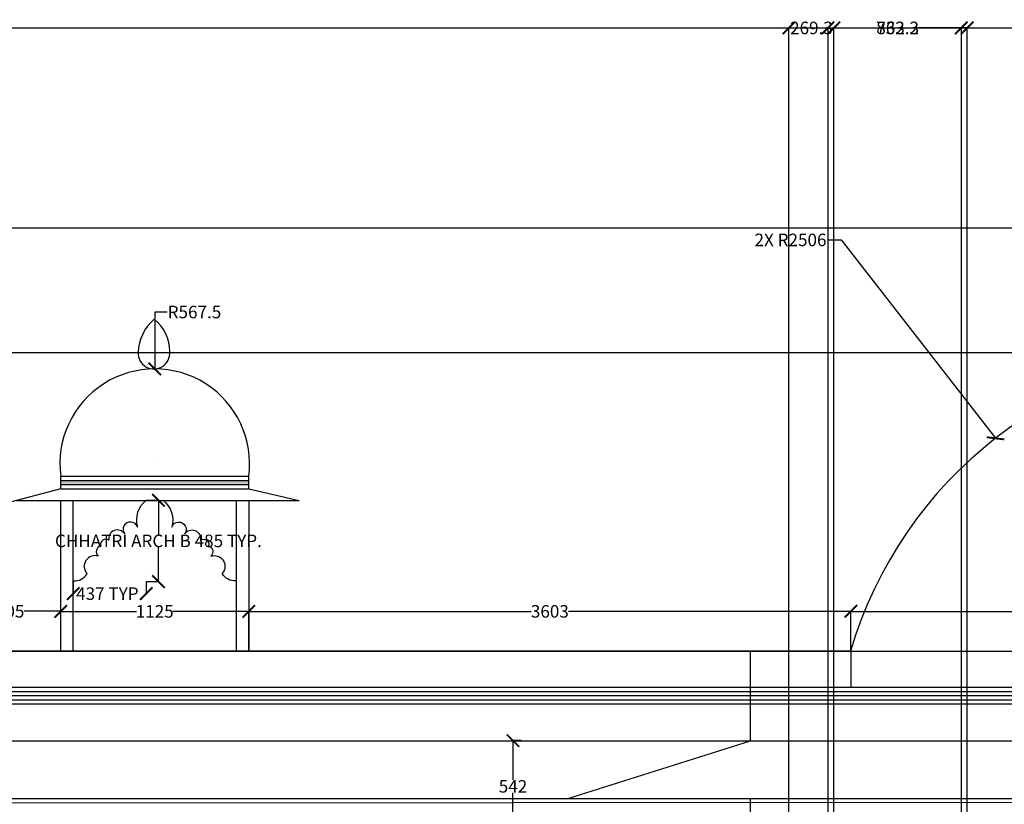
# Model space of a CAD drawing. Units: inches. Extents: x 829 to 33356404, y 1874 to 16983.
# Tile 5 of 9: x 4957 to 10848, y 12288 to 16983. Entities that reach past the tile are written whole.
import ezdxf

# ---------------------------------------------------------------- set-up
doc = ezdxf.new("R2010")
doc.units = ezdxf.units.IN
doc.header["$MEASUREMENT"] = 0
doc.header["$PDMODE"] = 3
for name, color, linetype, lineweight in [('A-ANNO-DIMS', 2, 'Continuous', 18), ('A-ELEV', 7, 'Continuous', 25), ('A-ELEV-PATT', 8, 'Continuous', 13)]:
    doc.layers.add(name, color=color, linetype=linetype, lineweight=lineweight)
doc.styles.get("Standard").update_dxf_attribs({"font": 'arial.ttf'})
doc.dimstyles.get("Standard").update_dxf_attribs({"dimtxt": 75, "dimasz": 75, "dimexe": 0.18, "dimexo": 0.0625, "dimgap": 0.09, "dimtad": 0, "dimtih": 1, "dimtoh": 1, "dimdec": 0, "dimzin": 0, "dimdsep": 46, "dimtxsty": 'Standard', "dimblk": 'ARCHTICK', "dimcen": 0.09, "dimadec": 0, "dimazin": 0, "dimtfac": 1, "dimtdec": 0, "dimtofl": 0, "dimtmove": 0, "dimatfit": 3, "dimfxl": 1, "dimtolj": 1, "dimtzin": 0, "dimarcsym": 0})

# ---------------------------------------------------------------- blocks, each defined once
blk = doc.blocks.new('_ArchTick')
at = {"color": 0, "linetype": 'ByBlock', "const_width": 0.15}
blk.add_lwpolyline([(-0.5, -0.5), (0.5, 0.5)], dxfattribs=at)
blk = doc.blocks.new('*D35')
at = {"layer": 'A-ANNO-DIMS', "color": 0, "lineweight": -2, "transparency": 16777216}
for p, q in [((7957.3, 12669.2), (7908.7, 12669.2)), ((7908.8, 12669.2), (7908.8, 12434.2)), ((7908.8, 12127.2), (7908.8, 12357.4)), ((7957.3, 12127.2), (7908.7, 12127.2))]:
    blk.add_line(p, q, dxfattribs=at)
at = {"layer": 'Defpoints', "color": 0, "transparency": 16777216}
for p in [(7908.8, 12669.2), (7957.3, 12669.2), (7957.3, 12127.2)]:
    blk.add_point(p, dxfattribs=at)
at = {"layer": 'A-ANNO-DIMS', "color": 0, "lineweight": -2, "transparency": 16777216, "xscale": 75, "yscale": 75, "zscale": 75}
for p, rotation in [((7908.8, 12669.2), 90), ((7908.8, 12127.2), 270)]:
    blk.add_blockref('_ArchTick', p, dxfattribs=dict(at, rotation=rotation))
at = {"layer": 'A-ANNO-DIMS', "color": 0, "transparency": 16777216, "insert": (7908.8, 12395.8), "char_height": 75, "attachment_point": 5}
blk.add_mtext('\\A1;542', dxfattribs=at)
blk = doc.blocks.new('*D47')
at = {"layer": 'A-ANNO-DIMS', "color": 0, "lineweight": -2, "transparency": 16777216}
for p, q in [((4597.8, 13204.1), (4597.8, 13443.2)), ((4597.8, 13443), (4816.8, 13443)), ((5202.8, 13443), (4983.7, 13443)), ((5202.8, 13204.1), (5202.8, 13443.2))]:
    blk.add_line(p, q, dxfattribs=at)
at = {"layer": 'Defpoints', "color": 0, "transparency": 16777216}
for p in [(5202.8, 13443), (4597.8, 13204), (5202.8, 13204)]:
    blk.add_point(p, dxfattribs=at)
at = {"layer": 'A-ANNO-DIMS', "color": 0, "lineweight": -2, "transparency": 16777216, "xscale": 75, "yscale": 75, "zscale": 75, "rotation": 180}
blk.add_blockref('_ArchTick', (4597.8, 13443), dxfattribs=at)
at = {"layer": 'A-ANNO-DIMS', "color": 0, "lineweight": -2, "transparency": 16777216, "xscale": 75, "yscale": 75, "zscale": 75}
blk.add_blockref('_ArchTick', (5202.8, 13443), dxfattribs=at)
at = {"layer": 'A-ANNO-DIMS', "color": 0, "transparency": 16777216, "insert": (4900.3, 13443), "char_height": 75, "attachment_point": 5}
blk.add_mtext('\\A1;605', dxfattribs=at)
blk = doc.blocks.new('*D48')
at = {"layer": 'A-ANNO-DIMS', "color": 0, "lineweight": -2, "transparency": 16777216}
for p, q in [((5202.8, 13273.1), (5202.8, 13442.8)), ((5202.8, 13442.7), (5656.4, 13442.7)), ((6327.8, 13442.7), (5874.1, 13442.7)), ((6327.8, 13273.1), (6327.8, 13442.8))]:
    blk.add_line(p, q, dxfattribs=at)
at = {"layer": 'Defpoints', "color": 0, "transparency": 16777216}
for p in [(6327.8, 13442.7), (5202.8, 13273), (6327.8, 13273)]:
    blk.add_point(p, dxfattribs=at)
at = {"layer": 'A-ANNO-DIMS', "color": 0, "lineweight": -2, "transparency": 16777216, "xscale": 75, "yscale": 75, "zscale": 75, "rotation": 180}
blk.add_blockref('_ArchTick', (5202.8, 13442.7), dxfattribs=at)
at = {"layer": 'A-ANNO-DIMS', "color": 0, "lineweight": -2, "transparency": 16777216, "xscale": 75, "yscale": 75, "zscale": 75}
blk.add_blockref('_ArchTick', (6327.8, 13442.7), dxfattribs=at)
at = {"layer": 'A-ANNO-DIMS', "color": 0, "transparency": 16777216, "insert": (5765.3, 13442.7), "char_height": 75, "attachment_point": 5}
blk.add_mtext('\\A1;1125', dxfattribs=at)
blk = doc.blocks.new('*D54')
at = {"layer": 'A-ANNO-DIMS', "color": 0, "lineweight": -2, "transparency": 16777216}
for p, q in [((6327.8, 13204.1), (6327.8, 13443)), ((6327.8, 13442.8), (8017.2, 13442.8)), ((9930.8, 13442.8), (8241.3, 13442.8)), ((9930.8, 13204.1), (9930.8, 13443))]:
    blk.add_line(p, q, dxfattribs=at)
at = {"layer": 'Defpoints', "color": 0, "transparency": 16777216}
for p in [(9930.8, 13442.8), (6327.8, 13204), (9930.8, 13204)]:
    blk.add_point(p, dxfattribs=at)
at = {"layer": 'A-ANNO-DIMS', "color": 0, "lineweight": -2, "transparency": 16777216, "xscale": 75, "yscale": 75, "zscale": 75, "rotation": 180}
blk.add_blockref('_ArchTick', (6327.8, 13442.8), dxfattribs=at)
at = {"layer": 'A-ANNO-DIMS', "color": 0, "lineweight": -2, "transparency": 16777216, "xscale": 75, "yscale": 75, "zscale": 75}
blk.add_blockref('_ArchTick', (9930.8, 13442.8), dxfattribs=at)
at = {"layer": 'A-ANNO-DIMS', "color": 0, "transparency": 16777216, "insert": (8129.3, 13442.8), "char_height": 75, "attachment_point": 5}
blk.add_mtext('\\A1;3603', dxfattribs=at)
blk = doc.blocks.new('*D55')
at = {"layer": 'A-ANNO-DIMS', "color": 0, "lineweight": -2, "transparency": 16777216}
for p, q in [((9930.8, 13204.1), (9930.8, 13443)), ((9930.8, 13442.8), (13449.1, 13442.8)), ((17190.8, 13442.8), (13672.4, 13442.8)), ((17190.8, 13204.1), (17190.8, 13443))]:
    blk.add_line(p, q, dxfattribs=at)
at = {"layer": 'Defpoints', "color": 0, "transparency": 16777216}
for p in [(17190.8, 13442.8), (9930.8, 13204), (17190.8, 13204)]:
    blk.add_point(p, dxfattribs=at)
at = {"layer": 'A-ANNO-DIMS', "color": 0, "lineweight": -2, "transparency": 16777216, "xscale": 75, "yscale": 75, "zscale": 75, "rotation": 180}
blk.add_blockref('_ArchTick', (9930.8, 13442.8), dxfattribs=at)
at = {"layer": 'A-ANNO-DIMS', "color": 0, "lineweight": -2, "transparency": 16777216, "xscale": 75, "yscale": 75, "zscale": 75}
blk.add_blockref('_ArchTick', (17190.8, 13442.8), dxfattribs=at)
at = {"layer": 'A-ANNO-DIMS', "color": 0, "transparency": 16777216, "insert": (13560.8, 13442.8), "char_height": 75, "attachment_point": 5}
blk.add_mtext('\\A1;7260', dxfattribs=at)
blk = doc.blocks.new('CHHATRI-ARCH-B')
blk.add_lwpolyline([(0, 0.5, 0.306755), (82.5, 43.8, 10.100933)], format="xyb")
for centre, radius, start, end in [((524.9, 364.6), 146.9, 126.85279, 196.90759), ((264.3, 252.9), 51.8, 32.98834, 190.27791), ((342.3, 308.5), 44.1, 17.62677, 218.36127), ((195.1, 217.8), 31.7, 54.88866, 193.78992), ((174.5, 175.2), 36.4, 106.30777, 227.87761), ((130.5, 86.8), 64.5, 72.31695, 221.86505)]:
    blk.add_arc(centre, radius, start, end)
blk = doc.blocks.new('*D76')
at = {"layer": 'A-ANNO-DIMS', "color": 0, "lineweight": -2, "transparency": 16777216}
for p, q in [((5714.6, 14107.2), (5787.6, 14107.2)), ((5787.4, 14107.2), (5787.4, 13903.3)), ((5787.4, 13621.7), (5787.4, 13825.6)), ((5714.6, 13621.7), (5787.6, 13621.7))]:
    blk.add_line(p, q, dxfattribs=at)
at = {"layer": 'Defpoints', "color": 0, "transparency": 16777216}
for p in [(5714.6, 14107.2), (5787.4, 14107.2), (5714.6, 13621.7)]:
    blk.add_point(p, dxfattribs=at)
at = {"layer": 'A-ANNO-DIMS', "color": 0, "lineweight": -2, "transparency": 16777216, "xscale": 75, "yscale": 75, "zscale": 75}
for p, rotation in [((5787.4, 14107.2), 90), ((5787.4, 13621.7), 270)]:
    blk.add_blockref('_ArchTick', p, dxfattribs=dict(at, rotation=rotation))
at = {"layer": 'A-ANNO-DIMS', "color": 0, "transparency": 16777216, "insert": (5787.4, 13864.5), "char_height": 75, "attachment_point": 5}
blk.add_mtext('\\A1;CHHATRI ARCH B 485 TYP.', dxfattribs=at)
blk = doc.blocks.new('*D77')
at = {"layer": 'A-ANNO-DIMS', "color": 0, "lineweight": -2, "transparency": 16777216}
for p, q in [((5277.8, 13621.7), (5277.8, 13548.7)), ((5714.6, 13621.7), (5714.6, 13548.7)), ((5277.8, 13548.9), (5282.9, 13548.9)), ((5714.6, 13548.9), (5709.4, 13548.9))]:
    blk.add_line(p, q, dxfattribs=at)
at = {"layer": 'Defpoints', "color": 0, "transparency": 16777216}
for p in [(5277.8, 13621.7), (5714.6, 13621.7), (5714.6, 13548.9)]:
    blk.add_point(p, dxfattribs=at)
at = {"layer": 'A-ANNO-DIMS', "color": 0, "lineweight": -2, "transparency": 16777216, "xscale": 75, "yscale": 75, "zscale": 75, "rotation": 180}
blk.add_blockref('_ArchTick', (5277.8, 13548.9), dxfattribs=at)
at = {"layer": 'A-ANNO-DIMS', "color": 0, "lineweight": -2, "transparency": 16777216, "xscale": 75, "yscale": 75, "zscale": 75}
blk.add_blockref('_ArchTick', (5714.6, 13548.9), dxfattribs=at)
at = {"layer": 'A-ANNO-DIMS', "color": 0, "transparency": 16777216, "insert": (5496.2, 13548.9), "char_height": 75, "attachment_point": 5}
blk.add_mtext('\\A1;437 TYP.', dxfattribs=at)
blk = doc.blocks.new('*D82')
at = {"layer": 'A-ANNO-DIMS', "color": 0, "lineweight": -2, "transparency": 16777216}
for p, q in [((2145.7, 12292.3), (2145.7, 16934.2)), ((2145.7, 16934), (13417.9, 16934)), ((24973.9, 16934), (13701.7, 16934)), ((24973.9, 12320.9), (24973.9, 16934.2))]:
    blk.add_line(p, q, dxfattribs=at)
at = {"layer": 'Defpoints', "color": 0, "transparency": 16777216}
for p in [(24973.9, 16934), (24973.9, 12320.9), (2145.7, 12292.2)]:
    blk.add_point(p, dxfattribs=at)
at = {"layer": 'A-ANNO-DIMS', "color": 0, "lineweight": -2, "transparency": 16777216, "xscale": 75, "yscale": 75, "zscale": 75, "rotation": 180}
blk.add_blockref('_ArchTick', (2145.7, 16934), dxfattribs=at)
at = {"layer": 'A-ANNO-DIMS', "color": 0, "lineweight": -2, "transparency": 16777216, "xscale": 75, "yscale": 75, "zscale": 75}
blk.add_blockref('_ArchTick', (24973.9, 16934), dxfattribs=at)
at = {"layer": 'A-ANNO-DIMS', "color": 0, "transparency": 16777216, "insert": (13559.8, 16934), "char_height": 75, "attachment_point": 5}
blk.add_mtext('\\A1;22828', dxfattribs=at)
blk = doc.blocks.new('*D83')
at = {"layer": 'A-ANNO-DIMS', "color": 0, "lineweight": -2, "transparency": 16777216}
for p, q in [((13604.5, 15734.9), (985.4, 15734.9)), ((985.6, 15734.9), (985.6, 10279.1)), ((985.6, 4746.5), (985.6, 10202.3)), ((3169.7, 4746.5), (985.4, 4746.5))]:
    blk.add_line(p, q, dxfattribs=at)
at = {"layer": 'Defpoints', "color": 0, "transparency": 16777216}
for p in [(985.6, 15734.9), (13604.5, 15734.9), (3169.8, 4746.5)]:
    blk.add_point(p, dxfattribs=at)
at = {"layer": 'A-ANNO-DIMS', "color": 0, "lineweight": -2, "transparency": 16777216, "xscale": 75, "yscale": 75, "zscale": 75}
for p, rotation in [((985.6, 15734.9), 90), ((985.6, 4746.5), 270)]:
    blk.add_blockref('_ArchTick', p, dxfattribs=dict(at, rotation=rotation))
at = {"layer": 'A-ANNO-DIMS', "color": 0, "transparency": 16777216, "insert": (985.6, 10240.7), "char_height": 75, "attachment_point": 5}
blk.add_mtext('\\A1;10988', dxfattribs=at)
blk = doc.blocks.new('*D84')
at = {"layer": 'A-ANNO-DIMS', "color": 0, "lineweight": -2, "transparency": 16777216}
for p, q in [((12044.3, 14988.9), (985.4, 14988.9)), ((985.6, 14988.9), (985.6, 14134.8)), ((985.6, 13204), (985.6, 14058.1)), ((9930.7, 13204), (985.4, 13204))]:
    blk.add_line(p, q, dxfattribs=at)
at = {"layer": 'Defpoints', "color": 0, "transparency": 16777216}
for p in [(985.6, 14988.9), (12044.4, 14988.9), (9930.8, 13204)]:
    blk.add_point(p, dxfattribs=at)
at = {"layer": 'A-ANNO-DIMS', "color": 0, "lineweight": -2, "transparency": 16777216, "xscale": 75, "yscale": 75, "zscale": 75}
for p, rotation in [((985.6, 14988.9), 90), ((985.6, 13204), 270)]:
    blk.add_blockref('_ArchTick', p, dxfattribs=dict(at, rotation=rotation))
at = {"layer": 'A-ANNO-DIMS', "color": 0, "transparency": 16777216, "insert": (985.6, 14096.5), "char_height": 75, "attachment_point": 5}
blk.add_mtext('\\A1;1785', dxfattribs=at)
blk = doc.blocks.new('*D105')
at = {"layer": 'A-ANNO-DIMS', "color": 0, "lineweight": -2, "transparency": 16777216}
for p, q in [((9829.2, 11877.3), (9829.2, 16934.2)), ((9829.2, 16934), (10084, 16934)), ((10591.5, 16934), (10336.6, 16934)), ((10591.5, 11877.3), (10591.5, 16934.2))]:
    blk.add_line(p, q, dxfattribs=at)
at = {"layer": 'Defpoints', "color": 0, "transparency": 16777216}
for p in [(10591.5, 16934), (9829.2, 11877.2), (10591.5, 11877.2)]:
    blk.add_point(p, dxfattribs=at)
at = {"layer": 'A-ANNO-DIMS', "color": 0, "lineweight": -2, "transparency": 16777216, "xscale": 75, "yscale": 75, "zscale": 75, "rotation": 180}
blk.add_blockref('_ArchTick', (9829.2, 16934), dxfattribs=at)
at = {"layer": 'A-ANNO-DIMS', "color": 0, "lineweight": -2, "transparency": 16777216, "xscale": 75, "yscale": 75, "zscale": 75}
blk.add_blockref('_ArchTick', (10591.5, 16934), dxfattribs=at)
at = {"layer": 'A-ANNO-DIMS', "color": 0, "transparency": 16777216, "insert": (10210.3, 16934), "char_height": 75, "attachment_point": 5}
blk.add_mtext('\\A1;762.3', dxfattribs=at)
blk = doc.blocks.new('*D106')
at = {"layer": 'A-ANNO-DIMS', "color": 0, "lineweight": -2, "transparency": 16777216}
for p, q in [((9559.8, 12127.3), (9559.8, 16934.2)), ((9559.8, 16934), (9567.2, 16934)), ((9829.2, 16934), (9821.8, 16934)), ((9829.2, 11877.3), (9829.2, 16934.2))]:
    blk.add_line(p, q, dxfattribs=at)
at = {"layer": 'Defpoints', "color": 0, "transparency": 16777216}
for p in [(9829.2, 16934), (9559.8, 12127.2), (9829.2, 11877.2)]:
    blk.add_point(p, dxfattribs=at)
at = {"layer": 'A-ANNO-DIMS', "color": 0, "lineweight": -2, "transparency": 16777216, "xscale": 75, "yscale": 75, "zscale": 75, "rotation": 180}
blk.add_blockref('_ArchTick', (9559.8, 16934), dxfattribs=at)
at = {"layer": 'A-ANNO-DIMS', "color": 0, "lineweight": -2, "transparency": 16777216, "xscale": 75, "yscale": 75, "zscale": 75}
blk.add_blockref('_ArchTick', (9829.2, 16934), dxfattribs=at)
at = {"layer": 'A-ANNO-DIMS', "color": 0, "transparency": 16777216, "insert": (9694.5, 16934), "char_height": 75, "attachment_point": 5}
blk.add_mtext('\\A1;269.3', dxfattribs=at)
blk = doc.blocks.new('*D107')
at = {"layer": 'A-ANNO-DIMS', "color": 0, "lineweight": -2, "transparency": 16777216}
for p, q in [((9793.7, 9982.3), (9793.7, 16934.2)), ((9793.7, 16934), (10084, 16934)), ((10626.9, 16934), (10336.6, 16934)), ((10626.9, 9982.3), (10626.9, 16934.2))]:
    blk.add_line(p, q, dxfattribs=at)
at = {"layer": 'Defpoints', "color": 0, "transparency": 16777216}
for p in [(10626.9, 16934), (9793.7, 9982.2), (10626.9, 9982.2)]:
    blk.add_point(p, dxfattribs=at)
at = {"layer": 'A-ANNO-DIMS', "color": 0, "lineweight": -2, "transparency": 16777216, "xscale": 75, "yscale": 75, "zscale": 75, "rotation": 180}
blk.add_blockref('_ArchTick', (9793.7, 16934), dxfattribs=at)
at = {"layer": 'A-ANNO-DIMS', "color": 0, "lineweight": -2, "transparency": 16777216, "xscale": 75, "yscale": 75, "zscale": 75}
blk.add_blockref('_ArchTick', (10626.9, 16934), dxfattribs=at)
at = {"layer": 'A-ANNO-DIMS', "color": 0, "transparency": 16777216, "insert": (10210.3, 16934), "char_height": 75, "attachment_point": 5}
blk.add_mtext('\\A1;833.2', dxfattribs=at)
blk = doc.blocks.new('*D109')
at = {"layer": 'A-ANNO-DIMS', "color": 0, "lineweight": -2, "transparency": 16777216}
for p, q in [((9798.3, 15665.5), (9873.3, 15665.5)), ((9873.3, 15665.5), (10796, 14478.3)), ((12333.6, 12499.6), (12333.8, 12499.6)), ((12333.7, 12499.5), (12333.7, 12499.7))]:
    blk.add_line(p, q, dxfattribs=at)
at = {"layer": 'Defpoints', "color": 0, "transparency": 16777216}
for p in [(10796, 14478.3), (12333.7, 12499.6)]:
    blk.add_point(p, dxfattribs=at)
at = {"layer": 'A-ANNO-DIMS', "color": 0, "lineweight": -2, "transparency": 16777216, "xscale": 75, "yscale": 75, "zscale": 75, "rotation": 307.8527471709181}
blk.add_blockref('_ArchTick', (10796, 14478.3), dxfattribs=at)
at = {"layer": 'A-ANNO-DIMS', "color": 0, "transparency": 16777216, "insert": (9569.2, 15665.5), "char_height": 75, "attachment_point": 5}
blk.add_mtext('\\A1;2X R2506', dxfattribs=at)
blk = doc.blocks.new('*D117')
at = {"layer": 'A-ANNO-DIMS', "color": 0, "lineweight": -2, "transparency": 16777216}
for p, q in [((5840.3, 15234), (5765.3, 15234)), ((5765.3, 15234), (5765.3, 14893.5)), ((5765.2, 14326), (5765.4, 14326)), ((5765.3, 14326), (5765.3, 14326.1))]:
    blk.add_line(p, q, dxfattribs=at)
at = {"layer": 'Defpoints', "color": 0, "transparency": 16777216}
for p in [(5765.3, 14893.5), (5765.3, 14326)]:
    blk.add_point(p, dxfattribs=at)
at = {"layer": 'A-ANNO-DIMS', "color": 0, "lineweight": -2, "transparency": 16777216, "xscale": 75, "yscale": 75, "zscale": 75, "rotation": 270}
blk.add_blockref('_ArchTick', (5765.3, 14893.5), dxfattribs=at)
at = {"layer": 'A-ANNO-DIMS', "color": 0, "transparency": 16777216, "insert": (6003.1, 15234), "char_height": 75, "attachment_point": 5}
blk.add_mtext('\\A1;R567.5', dxfattribs=at)

msp = doc.modelspace()

# ---------------------------------------------------------------- hatches: boundary and pattern name
at = {"layer": 'A-ELEV-PATT'}
h = msp.add_hatch(color=256, dxfattribs=at)
h.dxf.hatch_style = 1
h.paths.add_polyline_path([(5765.278, 14226.035), (5202.778, 14226.035), (5202.778, 14201.035), (5765.278, 14201.035)])
h = msp.add_hatch(color=256, dxfattribs=at)
h.dxf.hatch_style = 1
h.paths.add_polyline_path([(6327.778, 14226.035), (5765.278, 14226.035), (5765.278, 14201.035), (6327.778, 14201.035)])

# ---------------------------------------------------------------- linework, layer by layer
at = {"layer": 'A-ELEV'}
for p, q in [((5202.778, 14251.035), (6327.778, 14251.035)), ((5202.778, 14176.035), (5202.778, 14251.035)), ((5202.778, 14226.035), (6327.778, 14226.035)), ((5202.778, 14201.035), (6327.778, 14201.035)), ((6327.778, 14176.035), (6327.778, 14251.035)), ((5202.778, 14176.035), (4899.778, 14096.847)), ((5202.778, 14176.035), (6327.778, 14176.035)), ((6327.778, 14176.035), (6629.778, 14107.179)), ((4939.313, 14107.179), (6629.778, 14107.179)), ((5202.778, 13273.035), (5202.778, 14107.179)), ((5277.778, 13204.032), (5277.778, 14107.179)), ((6252.778, 14107.179), (6252.778, 13204.032)), ((6327.778, 14107.179), (6327.778, 13204.032)), ((3169.778, 13204.032), (23949.778, 13204.032)), ((9329.778, 12669.032), (9329.778, 13204.032)), ((9930.778, 13204.032), (9930.778, 12986.532)), ((23949.778, 12986.532), (3169.778, 12986.532)), ((23949.778, 12961.532), (3169.778, 12961.532)), ((23949.778, 12936.532), (3169.778, 12936.532)), ((23949.778, 12911.532), (3169.778, 12911.532)), ((23949.778, 12886.532), (3169.778, 12886.532)), ((3169.778, 12669.032), (23949.778, 12669.032)), ((8230.382, 12320.882), (9329.778, 12669.032)), ((24973.929, 12320.882), (2145.628, 12320.882)), ((9329.778, 12202.212), (9329.778, 12320.882)), ((24973.929, 12310.744), (2145.651, 12292.214))]:
    msp.add_line(p, q, dxfattribs=at)
for points in [[(5854.823, 14996.786, 0.23550233), (5762.404, 15190.273, 0.2104826), (5665.498, 14993.513, 0.2342095)], [(5765.276, 14893.64, 0.00000292), (5765.278, 14893.639, 0.0000033), (5765.28, 14893.64)]]:
    msp.add_lwpolyline(points, format="xyb", dxfattribs=at)
for centre, radius, start, end in [((5760.277, 14988.424), 94.915, 176.9265679, 5.0541249), ((12333.736, 12499.606), 2506, 92.0310878, 163.6743952), ((5765.278, 14326.044), 567.479, 352.4045325, 187.5954675)]:
    msp.add_arc(centre, radius, start, end, dxfattribs=at)

# ---------------------------------------------------------------- block references
msp.add_blockref('CHHATRI-ARCH-B', (5277.778, 13625.062), dxfattribs=at)
at = {"layer": 'A-ELEV', "extrusion": (0, 0, -1), "zscale": -1}
msp.add_blockref('CHHATRI-ARCH-B', (-6251.778, 13625.062), dxfattribs=at)

# ---------------------------------------------------------------- dimensions: what is measured, and where the dimension line sits
at = {"layer": 'A-ANNO-DIMS'}
for base, p1, p2, override, picture, middle in [((24973.929, 16934.032), (2145.651, 12292.214), (24973.929, 12320.882), {"dimdec": 0, "dimlfac": 1, "dimrnd": 0, "dimzin": 0, "dimdsep": 46, "dimlunit": 2}, '*D82', (13559.79, 16934.032)), ((9829.151, 16934.032), (9559.826, 12127.212), (9829.151, 11877.212), {"dimdec": 1, "dimlfac": 1, "dimrnd": 0, "dimzin": 0, "dimdsep": 46, "dimlunit": 2}, '*D106', (9694.488, 16934.032)), ((10626.905, 16934.032), (9793.728, 9982.196), (10626.905, 9982.196), {"dimdec": 1, "dimlfac": 1, "dimrnd": 0, "dimzin": 0, "dimdsep": 46, "dimlunit": 2}, '*D107', (10210.317, 16934.032)), ((10591.482, 16934.032), (9829.151, 11877.212), (10591.482, 11877.212), {"dimdec": 1, "dimlfac": 1, "dimrnd": 0, "dimzin": 0, "dimdsep": 46, "dimlunit": 2}, '*D105', (10210.317, 16934.032)), ((5202.778, 13443.042), (4597.778, 13204.032), (5202.778, 13204.032), {"dimclrd": 0, "dimclre": 0, "dimclrt": 0}, '*D47', (4900.278, 13443.042)), ((6327.778, 13442.662), (5202.778, 13273.035), (6327.778, 13273.035), {"dimclrd": 0, "dimclre": 0, "dimclrt": 0}, '*D48', (5765.278, 13442.662)), ((9930.778, 13442.842), (6327.778, 13204.032), (9930.778, 13204.032), {"dimclrd": 0, "dimclre": 0, "dimclrt": 0}, '*D54', (8129.278, 13442.842)), ((17190.778, 13442.842), (9930.778, 13204.032), (17190.778, 13204.032), {"dimclrd": 0, "dimclre": 0, "dimclrt": 0}, '*D55', (13560.778, 13442.842))]:
    dim = msp.add_linear_dim(base=base, p1=p1, p2=p2, dimstyle='Standard', override=override, dxfattribs=at)
    dim.commit()
    dim.dimension.update_dxf_attribs({"geometry": picture, "text_midpoint": middle})
for base, p1, p2, picture, middle in [((985.628, 15734.879), (3169.778, 4746.468), (13604.527, 15734.879), '*D83', (985.628, 10240.673)), ((985.628, 14988.895), (9930.778, 13204.032), (12044.389, 14988.895), '*D84', (985.628, 14096.463))]:
    dim = msp.add_linear_dim(base=base, p1=p1, p2=p2, angle=90, dimstyle='Standard', override={"dimdec": 0, "dimlfac": 1, "dimrnd": 0, "dimzin": 0, "dimdsep": 46, "dimlunit": 2}, dxfattribs=at)
    dim.commit()
    dim.dimension.update_dxf_attribs({"geometry": picture, "text_midpoint": middle})
dim = msp.add_radius_dim(center=(12333.736, 12499.606), mpoint=(10795.968, 14478.32), text='2X <>', dimstyle='Standard', override={"dimdec": 0, "dimlfac": 1, "dimrnd": 0, "dimzin": 0, "dimdsep": 46, "dimlunit": 2}, dxfattribs=at)
dim.commit()
dim.dimension.update_dxf_attribs({"geometry": '*D109', "text_midpoint": (9569.151, 15665.548), "dimtype": 164})
dim = msp.add_radius_dim(center=(5765.278, 14326.044), mpoint=(5765.278, 14893.523), dimstyle='Standard', override={"dimdec": 1, "dimlfac": 1, "dimrnd": 0, "dimzin": 0, "dimdsep": 46, "dimlunit": 2}, dxfattribs=at)
dim.commit()
dim.dimension.update_dxf_attribs({"geometry": '*D117', "text_midpoint": (6003.081, 15234.01), "dimtype": 164})
dim = msp.add_linear_dim(base=(5787.374, 14107.179), p1=(5714.558, 13621.736), p2=(5714.558, 14107.179), angle=90, text='CHHATRI ARCH B <> TYP.', dimstyle='Standard', override={"dimdec": 0, "dimrnd": 0, "dimzin": 0, "dimlunit": 2}, dxfattribs=at)
dim.commit()
dim.dimension.update_dxf_attribs({"geometry": '*D76', "text_midpoint": (5787.374, 13864.457)})
dim = msp.add_linear_dim(base=(5714.558, 13548.919), p1=(5277.778, 13621.736), p2=(5714.558, 13621.736), text='<> TYP.', dimstyle='Standard', override={"dimdec": 0, "dimrnd": 0, "dimzin": 0, "dimlunit": 2}, dxfattribs=at)
dim.commit()
dim.dimension.update_dxf_attribs({"geometry": '*D77', "text_midpoint": (5496.168, 13548.919)})
dim = msp.add_linear_dim(base=(7908.831, 12669.212), p1=(7957.331, 12127.212), p2=(7957.331, 12669.212), angle=90, dimstyle='Standard', override={"dimclrd": 0, "dimclre": 0, "dimclrt": 0}, dxfattribs=at)
dim.commit()
dim.dimension.update_dxf_attribs({"geometry": '*D35', "text_midpoint": (7908.831, 12395.806), "dimtype": 160})

doc.saveas('drawing.dxf')
